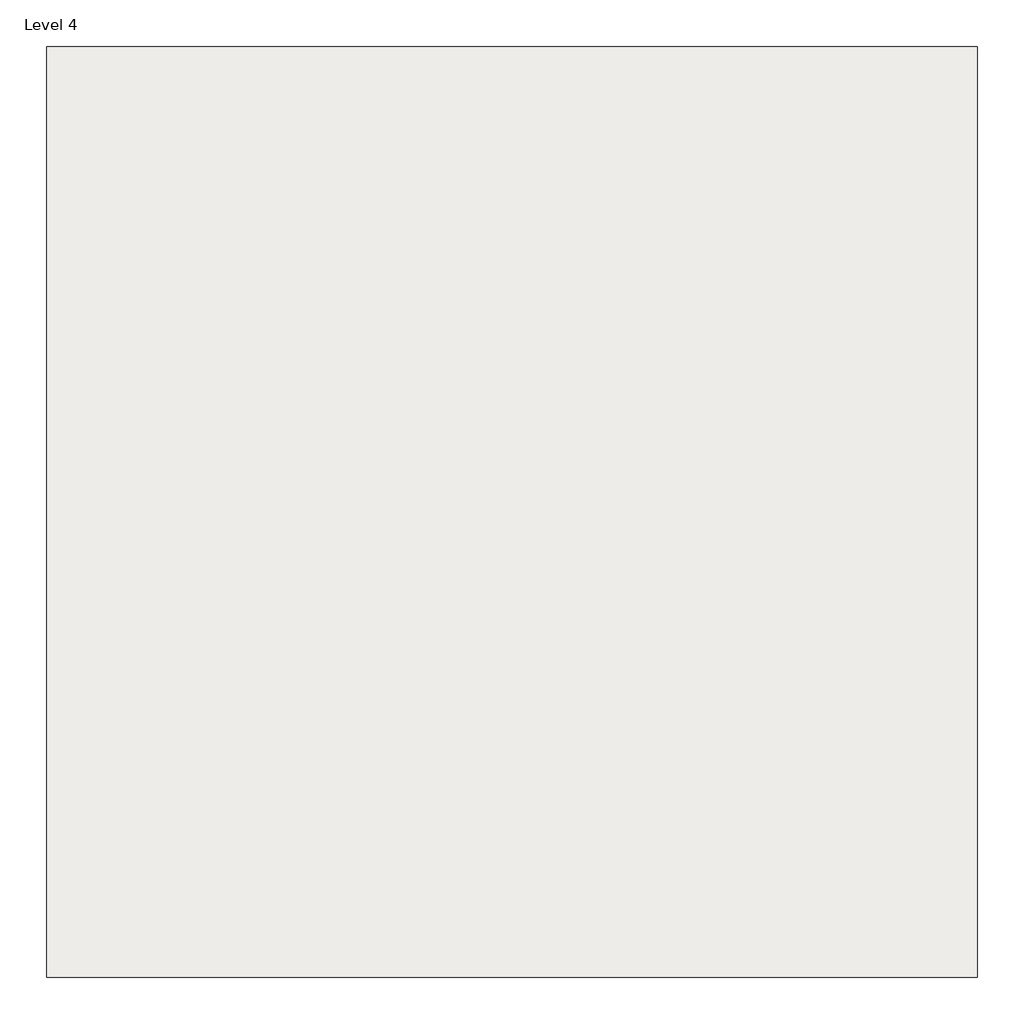
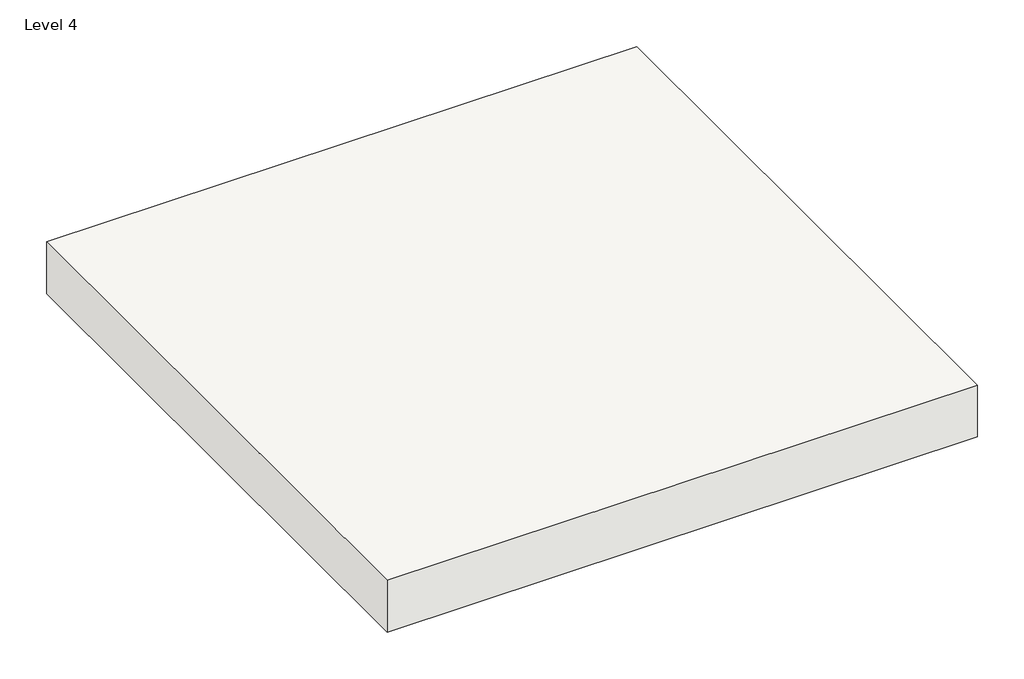
# One storey: 1 roof.
"""IFC4 building model written with IfcOpenShell, lengths in millimetres."""

from ifc_helpers import new_model, si_unit, frame, origin, place, context, project, spatial, polyline, outline, extrude, element, save

model = new_model("IFC4")

# Units and contexts
model_context = context("Model", 3, world=origin())
ifc_project = project(units=[si_unit("LENGTHUNIT", "METRE", prefix="MILLI")], contexts=[model_context])

# Site, building, storey
site = spatial("IfcSite", under=ifc_project)
building = spatial("IfcBuilding", under=site)
storey = spatial("IfcBuildingStorey", under=building, Name="Level 4", Elevation=10972.8)

# Roof
placement = place(None, origin())
element("IfcRoof", 1, ObjectType="Generic - 12\"", at=placement, inside=storey, context=model_context, shape_type="SweptSolid", body=[
    extrude(outline(polyline([(-5078.211895, 2347.1425923), (-1776.211895, 2347.1425923), (-1776.211895, -954.8574077), (-5078.211895, -954.8574077), (-5078.211895, 2347.1425923)])), frame((0.0, 0.0, 10972.8), z_axis=(0.0, 0.0, 1.0), x_axis=(1.0, 0.0, 0.0)), (0.0, 0.0, 1.0), 304.8),
])

save(model, "model.ifc")

# Revit data of these elements
# Type "Generic - 12\""
#   Assembly Code = "B1020"
#   Layers, outside or top first: 1' - 0" no material (function 1)
# Element 1 (IfcRoof, "Generic - 12\"")
#   built-in parameter 1001705 = 37 (stored number, unit not read)
#   built-in parameter 1001710 = 33615
#   Phase Created = New Construction
#   Materials on its faces: "Default Roof"
# Materials
#   "Default Roof": colour RGB 88 101 114, transparency 0
